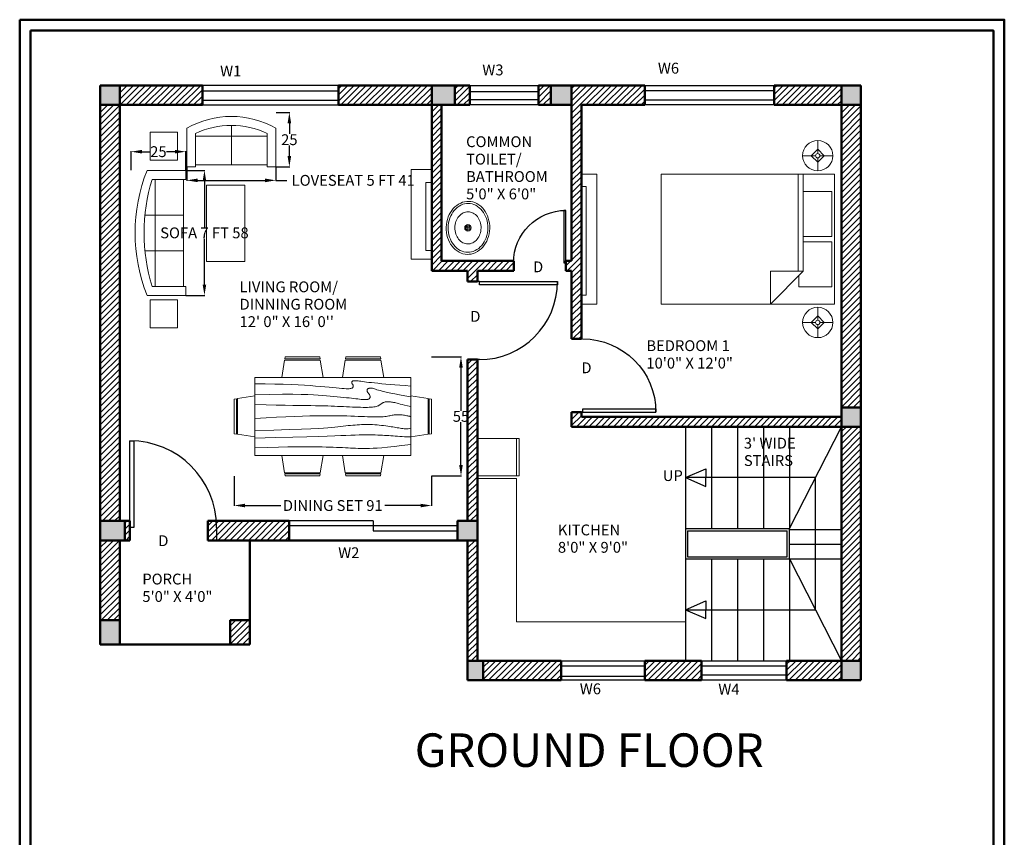
# Model space of a CAD drawing. Units: inches. Extents: x -25 to 429, y -18 to 847.
# Tile 3 of 3: x -25 to 429, y 470 to 847. Entities that reach past the tile are written whole.
import ezdxf

# ---------------------------------------------------------------- set-up
doc = ezdxf.new("R2010")
doc.units = ezdxf.units.IN
doc.header["$MEASUREMENT"] = 0
for name, color, linetype, lineweight in [('A-ANNO-DIMS', 2, 'Continuous', 18), ('A-ANNO-TEXT', 3, 'Continuous', 25), ('A-ANNO-TTLB', 7, 'Continuous', 50), ('A-AREA-IDEN', 7, 'Continuous', 25), ('A-DOOR', 4, 'Continuous', 25), ('A-FLOR-FIXT', 8, 'Continuous', 18), ('A-FLOR-STRS', 3, 'Continuous', 25), ('A-FURN', 8, 'Continuous', 18), ('A-GLAZ', 4, 'Continuous', 25), ('A-WALL', 7, 'Continuous', 50), ('A-WALL-FILL', 18, 'Continuous', 13), ('A-WALL-PATT', 252, 'Continuous', 13)]:
    doc.layers.add(name, color=color, linetype=linetype, lineweight=lineweight)
doc.styles.get("Standard").update_dxf_attribs({"font": 'arial.ttf'})
doc.dimstyles.get("Standard").update_dxf_attribs({"dimtxt": 5, "dimasz": 5, "dimexe": 0.18, "dimexo": 0.0625, "dimgap": 0.09, "dimtad": 0, "dimtih": 1, "dimtoh": 1, "dimdec": 1, "dimzin": 0, "dimdsep": 46, "dimlunit": 4, "dimtxsty": 'Standard', "dimcen": 0.09, "dimadec": 0, "dimazin": 0, "dimtfac": 1, "dimtdec": 1, "dimtofl": 0, "dimtmove": 0, "dimatfit": 3, "dimfxl": 1, "dimtolj": 1, "dimtzin": 0, "dimarcsym": 0})

# ---------------------------------------------------------------- blocks, each defined once
blk = doc.blocks.new('Sink - Oval top')
for p, q in [((-1, 0), (1, 0)), ((0, 1), (0, -1))]:
    blk.add_line(p, q)
for points in [[(-12.23, 0.39, 0.117634), (-11.46, -3.36, 0.104469), (-8.88, -6.8, 0.090016), (-5.08, -9.07, 0.08192), (-0.32, -10.02, 0.08192), (4.49, -9.38, 0.090016), (8.42, -7.36, 0.104469), (11.22, -4.09, 0.117634), (12.23, -0.39, 0.117634), (11.46, 3.36, 0.104469), (8.88, 6.8, 0.090016), (5.08, 9.07, 0.08192), (0.32, 10.02, 0.08192), (-4.49, 9.38, 0.090016), (-8.42, 7.36, 0.104469), (-11.22, 4.09, 0.117634)], [(-11.29, 0.16, 0.118622), (-10.52, -3.25, 0.104678), (-8.07, -6.36, 0.089562), (-4.54, -8.37, 0.081185), (-0.13, -9.15, 0.081185), (4.3, -8.49, 0.089562), (7.89, -6.58, 0.104678), (10.42, -3.55, 0.118622), (11.29, -0.16, 0.118622), (10.52, 3.25, 0.104678), (8.07, 6.36, 0.089562), (4.54, 8.37, 0.081185), (0.13, 9.15, 0.081185), (-4.3, 8.49, 0.089562), (-7.89, 6.58, 0.104678), (-10.42, 3.55, 0.118622)], [(-7.42, 0.08, 0.118283), (-6.91, -2.17, 0.104607), (-5.29, -4.21, 0.089718), (-2.97, -5.53, 0.081436), (-0.07, -6.04, 0.081436), (2.84, -5.59, 0.089718), (5.2, -4.33, 0.104607), (6.86, -2.32, 0.118283), (7.42, -0.08, 0.118283), (6.91, 2.17, 0.104607), (5.29, 4.21, 0.089718), (2.97, 5.53, 0.081436), (0.07, 6.04, 0.081436), (-2.84, 5.59, 0.089718), (-5.2, 4.33, 0.104607), (-6.86, 2.32, 0.118283)]]:
    blk.add_lwpolyline(points, format="xyb", close=True)
for radius in [1.5, 1]:
    blk.add_circle((0, 0), radius)
blk = doc.blocks.new('Bed - Queen')
for p, q in [((0, -80.00003), (0, 0)), ((0, 0), (59.99999, 0)), ((59.99999, 0), (59.99999, -80.00003)), ((7.99999, -1.2), (28.79998, -1.2)), ((7.99999, -14.4), (7.99999, -1.2)), ((28.79998, -1.2), (28.79998, -14.4)), ((31.19999, -1.2), (51.99999, -1.2)), ((31.19999, -14.4), (31.19999, -1.2)), ((51.99999, -1.2), (51.99999, -16.4)), ((0, -14.4), (44.8, -14.4)), ((44.8, -16.8), (0, -16.8)), ((59.99999, -29.6), (44.8, -14.4)), ((44.8, -14.4), (44.8, -29.6)), ((51.99999, -16.4), (46.79936, -16.4)), ((44.8, -29.6), (59.99999, -29.6)), ((59.99999, -80.00003), (0, -80.00003))]:
    blk.add_line(p, q)
blk = doc.blocks.new('Lamp - Table')
for p, q in [((0, 7), (0, 1)), ((-1, 0), (-7, 0)), ((0, 3), (-3, 0)), ((-3, 0), (0, -3)), ((3, 0), (0, 3)), ((0, -3), (3, 0)), ((1, 0), (7, 0)), ((0, -1), (0, -7))]:
    blk.add_line(p, q)
for radius in [7, 1]:
    blk.add_circle((0, 0), radius)
blk = doc.blocks.new('Sofa - Roundback 7 ft.')
for p, q in [((-12.00002, -32.4421), (-12.00003, -6.5971)), ((11.99997, -32.4421), (11.99998, -6.5971)), ((-36.000027, -34), (-36.000027, -11.4696)), ((35.99998, -34), (35.99998, -11.4696)), ((-35.999844, -13.3819), (35.9998, -13.3819)), ((-36.000027, -32.4421), (35.99998, -32.4421))]:
    blk.add_line(p, q)
for points in [[(-36.000027, -34), (-42.000027, -34), (-42.000027, -8)], [(41.99998, -8), (41.99998, -34), (35.99998, -34)]]:
    blk.add_lwpolyline(points)
for centre, radius, start, end in [((0, -114.25), 114.25, 68.43141, 111.5686), ((-0.00001, -127.1968), 121.1968, 72.72033, 107.2797)]:
    blk.add_arc(centre, radius, start, end)
blk = doc.blocks.new('Sofa - Roundback Loveseat 5 ft.')
for p, q in [((0, -32.44198), (0, -5.99998)), ((-24, -33.99998), (-24, -11.46958)), ((24.00004, -33.99998), (24.00004, -11.46958)), ((-23.9998, -13.38178), (23.99986, -13.38178)), ((-24, -32.44198), (24.00004, -32.44198))]:
    blk.add_line(p, q)
for points in [[(-24, -33.99998), (-30, -33.99998), (-30, -7.99998)], [(30.00004, -7.99998), (30.00004, -33.99998), (24.00004, -33.99998)]]:
    blk.add_lwpolyline(points)
for centre, radius, start, end in [((0, -60.24998), 60.24998, 60.13715, 119.8628), ((0, -61.38438), 55.38444, 64.32083, 115.6792)]:
    blk.add_arc(centre, radius, start, end)
blk = doc.blocks.new('Dining Set - 36 x 72 in.')
for p, q in [((-22, 27.5), (-22.1562, 26.50042)), ((-22, 27.5), (-6, 27.5)), ((-5.8437, 26.49966), (-6, 27.5)), ((6, 27.5), (5.8438, 26.50042)), ((6, 27.5), (22, 27.5)), ((22.1563, 26.49966), (22, 27.5)), ((-22.2343, 26.00059), (-23.4847, 17.99762)), ((-22.2304, 26), (-5.7608, 26)), ((-5.8416, 26.5), (-22.1534, 26.5)), ((-4.5152, 17.99762), (-5.7655, 25.99926)), ((5.7657, 26.00059), (4.5153, 17.99762)), ((5.7696, 26), (22.2392, 26)), ((22.1584, 26.5), (5.8466, 26.5)), ((23.4848, 17.99762), (22.2345, 25.99926)), ((36, 18), (-36, 18)), ((-36, 18), (-36, -18)), ((36, -18), (36, 18)), ((-44.0006, 8.23428), (-35.9976, 9.48474)), ((44.0006, 8.23428), (35.9976, 9.48474)), ((-45.5, 8), (-44.5004, 8.15617)), ((-45.5, 8), (-45.5, -8)), ((-44.5, -8.15843), (-44.5, 8.15338)), ((-44, 8.23041), (-44, -8.23915)), ((44, 8.23041), (44, -8.23915)), ((44.5, -8.15843), (44.5, 8.15338)), ((45.5, 8), (44.5005, 8.15617)), ((45.5, 8), (45.5, -8)), ((-44.4997, -8.15631), (-45.5, -8)), ((-35.9976, -9.48476), (-43.9993, -8.2345)), ((35.9976, -9.48476), (43.9993, -8.2345)), ((44.4997, -8.15631), (45.5, -8)), ((-36, -18), (36, -18)), ((-22.2343, -26.0006), (-23.4847, -17.99762)), ((-4.5152, -17.99762), (-5.7655, -25.99928)), ((5.7657, -26.0006), (4.5153, -17.99762)), ((23.4848, -17.99762), (22.2345, -25.99928)), ((-22.2304, -26), (-5.7608, -26)), ((-22, -27.5), (-22.1562, -26.50044)), ((-5.8416, -26.5), (-22.1534, -26.5)), ((-5.8437, -26.49967), (-6, -27.5)), ((5.7696, -26), (22.2392, -26)), ((6, -27.5), (5.8438, -26.50044)), ((22.1584, -26.5), (5.8466, -26.5)), ((22.1563, -26.49967), (22, -27.5)), ((-22, -27.5), (-6, -27.5)), ((6, -27.5), (22, -27.5))]:
    blk.add_line(p, q)
for points in [[(-36, 15), (-31.1772, 14.97754), (-26.8079, 14.91406), (-22.8538, 14.81543), (-19.276, 14.6875), (-16.0362, 14.53613), (-13.0957, 14.36718), (-10.4159, 14.18652), (-7.9583, 14), (-5.6904, 13.81315), (-3.6035, 13.63021), (-1.6954, 13.45508), (0.0365, 13.29166), (1.5945, 13.14388), (2.9811, 13.01562), (4.1988, 12.9108), (5.25, 12.83333), (6.1393, 12.78613), (6.8802, 12.76823), (7.4883, 12.77767), (7.9792, 12.8125), (8.3685, 12.87077), (8.6719, 12.95052), (8.9049, 13.0498), (9.0833, 13.16666), (9.2205, 13.29899), (9.3216, 13.44401), (9.3895, 13.59879), (9.4271, 13.76041), (9.4373, 13.92594), (9.4232, 14.09245), (9.3875, 14.257), (9.3333, 14.41666), (9.2638, 14.56917), (9.1836, 14.71484), (9.0975, 14.85465), (9.0104, 14.98958), (8.9272, 15.1206), (8.8529, 15.2487), (8.7922, 15.37483), (8.75, 15.5), (8.7305, 15.62467), (8.7344, 15.74739), (8.7617, 15.86621), (8.8125, 15.97916), (8.8867, 16.08431), (8.9844, 16.17968), (9.1055, 16.26334), (9.25, 16.33333), (9.4189, 16.38802), (9.6172, 16.42708), (9.8506, 16.45052), (10.125, 16.45833), (10.4463, 16.45052), (10.8203, 16.42708), (11.2529, 16.38802), (11.75, 16.33333), (12.3184, 16.26318), (12.9694, 16.17838), (13.7151, 16.07991), (14.5677, 15.96875), (15.5395, 15.84586), (16.6426, 15.71224), (17.8893, 15.56884), (19.2917, 15.41666), (20.859, 15.25667), (22.5879, 15.08984), (24.4721, 14.91715), (26.5052, 14.73958), (28.6809, 14.5581), (30.9929, 14.3737), (33.4347, 14.18733), (36, 14)], [(-36, 10), (-28.9766, 10.14274), (-23.1725, 10.20442), (-18.4241, 10.19775), (-14.5677, 10.13541), (-11.4399, 10.03011), (-8.877, 9.89453), (-6.7154, 9.74137), (-4.7917, 9.58333), (-2.9698, 9.43082), (-1.2246, 9.28515), (0.4415, 9.14534), (2.026, 9.01041), (3.5266, 8.87939), (4.9408, 8.7513), (6.266, 8.62516), (7.5, 8.5), (8.6411, 8.37549), (9.6914, 8.2539), (10.6538, 8.13818), (11.5312, 8.03125), (12.3267, 7.93603), (13.043, 7.85547), (13.6831, 7.79248), (14.25, 7.75), (14.7471, 7.7303), (15.1797, 7.73307), (15.5537, 7.75732), (15.875, 7.80208), (16.1494, 7.86637), (16.3828, 7.94922), (16.5811, 8.04964), (16.75, 8.16666), (16.8944, 8.29915), (17.0143, 8.44531), (17.1089, 8.60319), (17.1771, 8.77083), (17.218, 8.94629), (17.2305, 9.1276), (17.2137, 9.31282), (17.1667, 9.5), (17.0895, 9.6875), (16.987, 9.875), (16.8649, 10.0625), (16.7292, 10.25), (16.5856, 10.4375), (16.4401, 10.625), (16.2985, 10.8125), (16.1667, 11), (16.05, 11.18733), (15.9518, 11.3737), (15.8752, 11.5581), (15.8229, 11.73958), (15.798, 11.91715), (15.8034, 12.08984), (15.842, 12.25667), (15.9167, 12.41666), (16.0295, 12.56836), (16.1784, 12.70833), (16.3605, 12.83268), (16.5729, 12.9375), (16.8127, 13.01888), (17.0768, 13.07291), (17.3625, 13.0957), (17.6667, 13.08333), (17.9894, 13.03312), (18.3418, 12.94726), (18.7382, 12.82918), (19.1927, 12.68229), (19.7195, 12.51001), (20.3327, 12.31575), (21.0465, 12.10294), (21.875, 11.875), (22.8357, 11.63354), (23.959, 11.37304), (25.2786, 11.08618), (26.8282, 10.76562), (28.6414, 10.40405), (30.752, 9.99414), (33.1936, 9.52856), (36, 9)], [(-36, 5.5), (-30.7157, 5.3348), (-26.069, 5.20963), (-21.9946, 5.11767), (-18.4271, 5.05208), (-15.3009, 5.00602), (-12.5508, 4.97265), (-10.1112, 4.94515), (-7.9167, 4.91666), (-5.909, 4.88167), (-4.0586, 4.83984), (-2.3429, 4.79215), (-0.7396, 4.73958), (0.7739, 4.6831), (2.22, 4.6237), (3.6213, 4.56233), (5, 4.5), (6.373, 4.43782), (7.7344, 4.3776), (9.0723, 4.32129), (10.375, 4.27083), (11.6309, 4.22819), (12.8281, 4.19531), (13.9551, 4.17415), (15, 4.16666), (15.954, 4.17448), (16.819, 4.19791), (17.6001, 4.23698), (18.3021, 4.29166), (18.9299, 4.36198), (19.4883, 4.44791), (19.9823, 4.54948), (20.4167, 4.66666), (20.7969, 4.79899), (21.1302, 4.94401), (21.4245, 5.09879), (21.6875, 5.26041), (21.9271, 5.42594), (22.1511, 5.59245), (22.3672, 5.757), (22.5834, 5.91666), (22.8065, 6.06868), (23.0404, 6.21093), (23.2879, 6.34147), (23.5521, 6.45833), (23.8358, 6.55957), (24.142, 6.64323), (24.4735, 6.70735), (24.8334, 6.75), (25.2235, 6.76969), (25.642, 6.76692), (26.0858, 6.74267), (26.5521, 6.69791), (27.0379, 6.63362), (27.5404, 6.55078), (28.0565, 6.45036), (28.5834, 6.33333), (29.1242, 6.19987), (29.7071, 6.04687), (30.3661, 5.87044), (31.1354, 5.66666), (32.0493, 5.43164), (33.142, 5.16146), (34.4475, 4.85221), (36, 4.5)], [(-36, -1), (-30.7915, -0.6591), (-26.0195, -0.38216), (-21.6519, -0.16284), (-17.6563, 0.00521), (-14.0005, 0.12833), (-10.6523, 0.21289), (-7.5796, 0.26522), (-4.75, 0.29166), (-2.134, 0.29793), (0.2878, 0.28711), (2.5317, 0.26163), (4.6146, 0.22396), (6.5529, 0.17651), (8.3633, 0.12174), (10.0623, 0.06209), (11.6667, 0), (13.1899, -0.06201), (14.6341, -0.1211), (15.9982, -0.17432), (17.2813, -0.21875), (18.4823, -0.25147), (19.6003, -0.26953), (20.6343, -0.27002), (21.5834, -0.25), (22.4481, -0.20768), (23.2357, -0.14584), (23.9549, -0.06836), (24.6146, 0.02083), (25.2235, 0.11784), (25.7904, 0.21875), (26.3241, 0.31966), (26.8334, 0.41666), (27.3265, 0.50618), (27.8099, 0.58593), (28.2894, 0.65397), (28.7709, 0.70833), (29.2601, 0.74707), (29.763, 0.76823), (30.2855, 0.76985), (30.8334, 0.75), (31.4088, 0.70784), (31.9994, 0.64713), (32.589, 0.57275), (33.1615, 0.48958), (33.7008, 0.4025), (34.1908, 0.3164), (34.6153, 0.23616), (34.9584, 0.16666), (35.2099, 0.11165), (35.3848, 0.07031), (35.504, 0.04069), (35.5886, 0.02083), (35.6594, 0.00879), (35.7377, 0.0026), (35.8442, 0.00032), (36, 0)], [(-36, -6.5), (-27.1843, -6.31267), (-20.084, -6.1263), (-14.469, -5.9419), (-10.1094, -5.76042), (-6.7752, -5.58285), (-4.2363, -5.41016), (-2.2629, -5.24333), (-0.625, -5.08334), (0.8708, -4.93099), (2.2715, -4.78646), (3.5872, -4.64974), (4.8281, -4.52084), (6.0046, -4.39974), (7.127, -4.28646), (8.2053, -4.18099), (9.25, -4.08334), (10.2705, -3.99382), (11.2734, -3.91407), (12.2647, -3.84603), (13.25, -3.79167), (14.2354, -3.75293), (15.2266, -3.73177), (16.2295, -3.73015), (17.25, -3.75), (18.2912, -3.79248), (19.3451, -3.85547), (20.4009, -3.93604), (21.4479, -4.03125), (22.4754, -4.13819), (23.4727, -4.25391), (24.4289, -4.37549), (25.3334, -4.5), (26.1785, -4.62492), (26.9694, -4.74935), (27.7145, -4.87281), (28.4219, -4.99479), (29.1, -5.11483), (29.7572, -5.23242), (30.4016, -5.34709), (31.0417, -5.45834), (31.6837, -5.56437), (32.3262, -5.65821), (32.9658, -5.73153), (33.599, -5.77604), (34.2224, -5.78345), (34.8327, -5.74545), (35.4264, -5.65373), (36, -5.5)], [(-36, -10), (-26.4022, -9.81299), (-18.4675, -9.62891), (-11.9839, -9.45069), (-6.7396, -9.28125), (-2.5226, -9.12354), (0.8789, -8.98047), (3.6769, -8.85498), (6.0833, -8.75), (8.2767, -8.66765), (10.3021, -8.60677), (12.1712, -8.56543), (13.8958, -8.54167), (15.4876, -8.53353), (16.9583, -8.53907), (18.3197, -8.55632), (19.5834, -8.58334), (20.7616, -8.61841), (21.8685, -8.66081), (22.9188, -8.71004), (23.9271, -8.76563), (24.9081, -8.82707), (25.8763, -8.89388), (26.8465, -8.96558), (27.8334, -9.04167), (28.8474, -9.12118), (29.8828, -9.20117), (30.93, -9.27824), (31.9792, -9.34896), (33.0205, -9.40991), (34.0443, -9.45768), (35.0407, -9.48885), (36, -9.5)], [(-36, -14.5), (-30.0881, -14.33513), (-25.0332, -14.21224), (-20.7312, -14.12647), (-17.0781, -14.07292), (-13.97, -14.04671), (-11.3027, -14.04297), (-8.9724, -14.05681), (-6.875, -14.08334), (-4.9224, -14.11833), (-3.0905, -14.16016), (-1.3709, -14.20785), (0.2448, -14.26042), (1.7647, -14.3169), (3.1973, -14.3763), (4.5507, -14.43767), (5.8333, -14.5), (7.0554, -14.5621), (8.235, -14.62175), (9.3922, -14.67652), (10.5469, -14.72396), (11.7192, -14.76164), (12.929, -14.78711), (14.1965, -14.79794), (15.5417, -14.79167), (16.9933, -14.76424), (18.6152, -14.70508), (20.4804, -14.60197), (22.6615, -14.44271), (25.2312, -14.21509), (28.2624, -13.9069), (31.8277, -13.50594), (36, -13)]]:
    blk.add_lwpolyline(points)
blk = doc.blocks.new('*U10')
for p, q in [((0, 0), (0, -6)), ((40, 0), (40, -6))]:
    blk.add_line(p, q)
blk.add_lwpolyline([(0, 0), (0, 40), (1.75, 40), (1.75, 0)], close=True)
blk.add_arc((0, 0), 40, 0, 90)
blk = doc.blocks.new('*D21')
at = {"layer": 'A-ANNO-DIMS', "color": 0, "lineweight": -2, "ltscale": 0.5, "transparency": 16777216}
for p, q in [((51.61, 777.34), (60.37, 777.34)), ((60.19, 772.34), (60.19, 751.19)), ((60.19, 724.68), (60.19, 745.83)), ((51.61, 719.68), (60.37, 719.68))]:
    blk.add_line(p, q, dxfattribs=at)
at = {"layer": 'A-ANNO-DIMS', "color": 0, "lineweight": 100, "ltscale": 0.5, "transparency": 16777216}
for points in [[(59.36, 772.34), (61.03, 772.34), (60.19, 777.34)], [(59.36, 724.68), (61.03, 724.68), (60.19, 719.68)]]:
    blk.add_solid(points, dxfattribs=at)
at = {"layer": 'Defpoints', "color": 0, "lineweight": 100, "ltscale": 0.5, "transparency": 16777216}
for p in [(51.54, 777.34), (60.19, 777.34), (51.54, 719.68)]:
    blk.add_point(p, dxfattribs=at)
at = {"layer": 'A-ANNO-DIMS', "color": 0, "ltscale": 0.5, "transparency": 16777216, "insert": (60.19, 748.51), "char_height": 5, "attachment_point": 5}
blk.add_mtext('\\A1;SOFA 7 FT 58', dxfattribs=at)
blk = doc.blocks.new('*D22')
at = {"layer": 'A-ANNO-DIMS', "color": 0, "lineweight": -2, "ltscale": 0.5, "transparency": 16777216}
for p, q in [((26.37, 777.4), (26.37, 786.17)), ((51.54, 777.4), (51.54, 786.17)), ((31.37, 785.99), (35.23, 785.99)), ((46.54, 785.99), (42.69, 785.99))]:
    blk.add_line(p, q, dxfattribs=at)
at = {"layer": 'A-ANNO-DIMS', "color": 0, "lineweight": 100, "ltscale": 0.5, "transparency": 16777216}
for points in [[(31.37, 786.82), (31.37, 785.15), (26.37, 785.99)], [(46.54, 786.82), (46.54, 785.15), (51.54, 785.99)]]:
    blk.add_solid(points, dxfattribs=at)
at = {"layer": 'Defpoints', "color": 0, "lineweight": 100, "ltscale": 0.5, "transparency": 16777216}
for p in [(26.37, 785.99), (26.37, 777.34), (51.54, 777.34)]:
    blk.add_point(p, dxfattribs=at)
at = {"layer": 'A-ANNO-DIMS', "color": 0, "ltscale": 0.5, "transparency": 16777216, "insert": (38.96, 785.99), "char_height": 5, "attachment_point": 5}
blk.add_mtext('\\A1;25', dxfattribs=at)
blk = doc.blocks.new('*D25')
at = {"layer": 'A-ANNO-DIMS', "color": 0, "lineweight": -2, "ltscale": 0.5, "transparency": 16777216}
for p, q in [((52.02, 778.86), (52.02, 772.57)), ((93.2, 778.86), (93.2, 772.57)), ((57.02, 772.75), (88.2, 772.75)), ((93.2, 772.75), (98.2, 772.75))]:
    blk.add_line(p, q, dxfattribs=at)
at = {"layer": 'A-ANNO-DIMS', "color": 0, "lineweight": 100, "ltscale": 0.5, "transparency": 16777216}
for points in [[(57.02, 773.58), (57.02, 771.91), (52.02, 772.75)], [(88.2, 773.58), (88.2, 771.91), (93.2, 772.75)]]:
    blk.add_solid(points, dxfattribs=at)
at = {"layer": 'Defpoints', "color": 0, "lineweight": 100, "ltscale": 0.5, "transparency": 16777216}
for p in [(52.02, 778.93), (93.2, 778.93), (93.2, 772.75)]:
    blk.add_point(p, dxfattribs=at)
at = {"layer": 'A-ANNO-DIMS', "color": 0, "ltscale": 0.5, "transparency": 16777216, "insert": (128.84, 772.75), "char_height": 5, "attachment_point": 5}
blk.add_mtext('\\A1;LOVESEAT 5 FT 41', dxfattribs=at)
blk = doc.blocks.new('*D26')
at = {"layer": 'A-ANNO-DIMS', "color": 0, "lineweight": -2, "ltscale": 0.5, "transparency": 16777216}
for p, q in [((93.27, 804.1), (99.56, 804.1)), ((99.38, 799.1), (99.38, 794.15)), ((99.38, 783.93), (99.38, 788.87)), ((93.27, 778.93), (99.56, 778.93))]:
    blk.add_line(p, q, dxfattribs=at)
at = {"layer": 'A-ANNO-DIMS', "color": 0, "lineweight": 100, "ltscale": 0.5, "transparency": 16777216}
for points in [[(98.55, 799.1), (100.21, 799.1), (99.38, 804.1)], [(98.55, 783.93), (100.21, 783.93), (99.38, 778.93)]]:
    blk.add_solid(points, dxfattribs=at)
at = {"layer": 'Defpoints', "color": 0, "lineweight": 100, "ltscale": 0.5, "transparency": 16777216}
for p in [(93.2, 804.1), (99.38, 804.1), (93.2, 778.93)]:
    blk.add_point(p, dxfattribs=at)
at = {"layer": 'A-ANNO-DIMS', "color": 0, "ltscale": 0.5, "transparency": 16777216, "insert": (99.38, 791.51), "char_height": 5, "attachment_point": 5}
blk.add_mtext('\\A1;25', dxfattribs=at)
blk = doc.blocks.new('*D35')
at = {"layer": 'A-ANNO-DIMS', "color": 0, "lineweight": -2, "ltscale": 0.5, "transparency": 16777216}
for p, q in [((73.92, 636.24), (73.92, 622.48)), ((164.92, 636.24), (164.92, 622.48)), ((78.92, 622.66), (95.4, 622.66)), ((159.92, 622.66), (143.44, 622.66))]:
    blk.add_line(p, q, dxfattribs=at)
at = {"layer": 'A-ANNO-DIMS', "color": 0, "lineweight": 100, "ltscale": 0.5, "transparency": 16777216}
for points in [[(78.92, 623.49), (78.92, 621.82), (73.92, 622.66)], [(159.92, 623.49), (159.92, 621.82), (164.92, 622.66)]]:
    blk.add_solid(points, dxfattribs=at)
at = {"layer": 'Defpoints', "color": 0, "lineweight": 100, "ltscale": 0.5, "transparency": 16777216}
for p in [(73.92, 636.31), (164.92, 636.31), (164.92, 622.66)]:
    blk.add_point(p, dxfattribs=at)
at = {"layer": 'A-ANNO-DIMS', "color": 0, "ltscale": 0.5, "transparency": 16777216, "insert": (119.42, 622.66), "char_height": 5, "attachment_point": 5}
blk.add_mtext('\\A1;DINING SET 91', dxfattribs=at)
blk = doc.blocks.new('*D36')
at = {"layer": 'A-ANNO-DIMS', "color": 0, "lineweight": -2, "ltscale": 0.5, "transparency": 16777216}
for p, q in [((164.98, 691.31), (178.75, 691.31)), ((178.57, 686.31), (178.57, 666.44)), ((178.57, 641.31), (178.57, 661.17)), ((164.98, 636.31), (178.75, 636.31))]:
    blk.add_line(p, q, dxfattribs=at)
at = {"layer": 'A-ANNO-DIMS', "color": 0, "lineweight": 100, "ltscale": 0.5, "transparency": 16777216}
for points in [[(177.73, 686.31), (179.4, 686.31), (178.57, 691.31)], [(177.73, 641.31), (179.4, 641.31), (178.57, 636.31)]]:
    blk.add_solid(points, dxfattribs=at)
at = {"layer": 'Defpoints', "color": 0, "lineweight": 100, "ltscale": 0.5, "transparency": 16777216}
for p in [(164.92, 691.31), (178.57, 691.31), (164.92, 636.31)]:
    blk.add_point(p, dxfattribs=at)
at = {"layer": 'A-ANNO-DIMS', "color": 0, "ltscale": 0.5, "transparency": 16777216, "insert": (178.57, 663.81), "char_height": 5, "attachment_point": 5}
blk.add_mtext('\\A1;55', dxfattribs=at)

msp = doc.modelspace()

# ---------------------------------------------------------------- hatches: boundary and pattern name
at = {"layer": 'A-WALL-FILL', "ltscale": 0.5}
h = msp.add_hatch(color=256, dxfattribs=at)
h.dxf.hatch_style = 1
h.paths.add_polyline_path([(21.13, 816.54), (12.13, 816.54), (12.13, 807.54), (21.13, 807.54)])
h.paths.add_polyline_path([(175.79, 816.54), (165.13, 816.54), (165.13, 807.54), (175.79, 807.54)])
h.paths.add_polyline_path([(229.63, 816.54), (220.08, 816.54), (220.08, 807.54), (229.63, 807.54)])
h.paths.add_polyline_path([(363.13, 816.54), (354.13, 816.54), (354.13, 807.54), (357.13, 807.54), (363.13, 807.54)])
h.paths.add_polyline_path([(186.13, 615.54), (176.99, 615.54), (176.99, 606.54), (186.13, 606.54)])
h.paths.add_polyline_path([(23.44, 615.54), (12.13, 615.54), (12.13, 606.54), (23.44, 606.54)])
h.paths.add_polyline_path([(21.13, 569.73), (12.13, 569.73), (12.13, 558.54), (21.13, 558.54)])
h.paths.add_polyline_path([(188.77, 551.04), (181.63, 551.04), (181.63, 542.04), (188.77, 542.04)])
h.paths.add_polyline_path([(363.13, 551.04), (354.13, 551.04), (354.13, 542.04), (363.13, 542.04)])
h.paths.add_polyline_path([(363.13, 667.89), (354.13, 667.89), (354.13, 659.04), (363.13, 659.04)])
at = {"layer": 'A-WALL-PATT', "ltscale": 0.5}
h = msp.add_hatch(dxfattribs=at)
h.set_pattern_fill('ANSI31', color=256, scale=16)
h.paths.add_polyline_path([(21.13, 807.54), (12.13, 807.54), (12.13, 615.54), (21.13, 615.54)])
h.paths.add_polyline_path([(59.28, 816.54), (21.13, 816.54), (21.13, 807.54), (59.28, 807.54)])
h.paths.add_polyline_path([(165.13, 816.54), (122.04, 816.54), (122.04, 807.54), (165.13, 807.54)])
h.paths.add_polyline_path([(182.62, 816.54), (175.79, 816.54), (175.79, 807.54), (182.62, 807.54)])
h.paths.add_polyline_path([(220.08, 816.54), (214.31, 816.54), (214.31, 807.54), (220.08, 807.54)])
h.paths.add_polyline_path([(263.36, 816.54), (229.63, 816.54), (229.63, 807.54), (229.63, 735.54), (227.02, 735.54), (227.02, 731.04), (229.63, 731.04), (229.63, 699.54), (234.13, 699.54), (234.13, 807.54), (263.36, 807.54)])
h.paths.add_polyline_path([(169.63, 807.54), (165.13, 807.54), (165.13, 731.04), (181.63, 731.04), (181.63, 726.06), (186.13, 726.06), (186.13, 731.04), (203.02, 731.04), (203.02, 735.54), (169.63, 735.54)])
h.paths.add_polyline_path([(354.13, 816.54), (323.12, 816.54), (323.12, 807.54), (354.13, 807.54)])
h.paths.add_polyline_path([(363.13, 807.54), (354.13, 807.54), (354.13, 667.89), (363.13, 667.89)])
h.paths.add_polyline_path([(354.13, 663.54), (234.13, 663.54), (234.13, 665.73), (229.63, 665.73), (229.63, 659.04), (354.13, 659.04)])
h.paths.add_polyline_path([(363.13, 659.04), (354.13, 659.04), (354.13, 612.04), (354.13, 598.04), (354.13, 551.04), (363.13, 551.04)])
h.paths.add_polyline_path([(354.13, 551.04), (328.82, 551.04), (328.82, 542.04), (354.13, 542.04)])
h.paths.add_polyline_path([(289.58, 551.04), (263.34, 551.04), (263.34, 542.04), (289.58, 542.04)])
h.paths.add_polyline_path([(224.82, 551.04), (188.77, 551.04), (188.77, 542.04), (224.82, 542.04)])
h.paths.add_polyline_path([(186.13, 606.54), (181.63, 606.54), (181.63, 551.04), (186.13, 551.04)])
h.paths.add_polyline_path([(99.25, 615.54), (61.79, 615.54), (61.79, 606.54), (99.25, 606.54)])
h.paths.add_polyline_path([(81.13, 569.73), (72.13, 569.73), (72.13, 558.54), (81.13, 558.54)])
h.paths.add_polyline_path([(21.13, 606.54), (12.13, 606.54), (12.13, 569.73), (21.13, 569.73)])
h.paths.add_polyline_path([(25.79, 615.54), (23.44, 615.54), (23.44, 606.54), (25.79, 606.54)])
h.paths.add_polyline_path([(186.13, 690.06), (181.63, 690.06), (181.63, 615.54), (186.13, 615.54)])

# ---------------------------------------------------------------- linework, layer by layer
at = {"layer": 'A-ANNO-TTLB', "ltscale": 0.5}
for points in [[(-25.05, 846.91), (429.28, 846.91), (429.28, -17.53), (-25.05, -17.53)], [(-20.05, 841.91), (424.28, 841.91), (424.28, -12.53), (-20.05, -12.53)]]:
    msp.add_lwpolyline(points, close=True, dxfattribs=at)
at = {"layer": 'A-FLOR-FIXT', "ltscale": 0.5}
for p, q in [((204.13, 653.62), (205.46, 653.62)), ((205.46, 653.62), (205.46, 636.32)), ((205.46, 636.32), (204.13, 636.32)), ((186.13, 635.19), (204.13, 635.19)), ((204.13, 635.19), (204.13, 569.04)), ((204.13, 569.04), (282.13, 569.04))]:
    msp.add_line(p, q, dxfattribs=at)
msp.add_lwpolyline([(186.13, 636.37), (204.13, 636.37), (204.13, 653.62), (186.13, 653.62)], close=True, dxfattribs=at)
at = {"layer": 'A-FLOR-STRS'}
for p, q in [((282.13, 659.04), (282.13, 612.04)), ((282.13, 612.04), (282.13, 598.04)), ((283.13, 611.04), (283.13, 599.04)), ((282.13, 598.04), (282.13, 551.04))]:
    msp.add_line(p, q, dxfattribs=at)
at = {"layer": 'A-FLOR-STRS', "ltscale": 0.5}
for p, q in [((294.12, 659.04), (294.12, 612.04)), ((306.12, 659.04), (306.12, 612.04)), ((318.12, 659.04), (318.12, 612.04)), ((330.12, 659.04), (330.12, 612.04)), ((330.13, 612.04), (354.13, 659.04)), ((282.13, 635.54), (291.57, 639.63)), ((291.57, 639.63), (291.57, 635.54)), ((342.13, 635.54), (282.13, 635.54)), ((282.13, 635.54), (291.57, 631.46)), ((291.57, 631.46), (291.57, 635.54)), ((342.12, 574.54), (342.13, 635.54)), ((282.13, 612.04), (330.13, 612.04)), ((283.13, 611.04), (329.13, 611.04)), ((329.13, 599.04), (329.13, 611.04)), ((330.13, 599.04), (330.13, 612.04)), ((330.13, 611.04), (330.13, 612.04)), ((330.13, 611.54), (354.13, 611.54)), ((330.13, 604.88), (354.13, 604.88)), ((282.13, 598.04), (330.13, 598.04)), ((282.13, 598.04), (282.13, 551.04)), ((283.13, 599.04), (329.13, 599.04)), ((294.12, 598.04), (294.12, 551.04)), ((306.12, 598.04), (306.12, 551.04)), ((318.12, 598.04), (318.12, 551.04)), ((330.12, 598.04), (330.12, 551.04)), ((330.12, 598.04), (354.13, 551.04)), ((330.13, 598.04), (330.13, 599.04)), ((330.13, 598.04), (354.13, 598.04)), ((282.13, 574.54), (291.57, 578.63)), ((291.57, 578.63), (291.57, 574.54)), ((282.13, 574.54), (342.12, 574.54)), ((282.13, 574.54), (291.57, 570.46)), ((291.57, 570.46), (291.57, 574.54))]:
    msp.add_line(p, q, dxfattribs=at)
at = {"layer": 'A-FURN'}
for points in [[(47.84, 782.11), (35.08, 782.11), (35.08, 794.96), (47.84, 794.96)], [(78.87, 735.31), (61.13, 735.31), (61.13, 770.47), (78.87, 770.47)], [(47.84, 704.68), (35.08, 704.68), (35.08, 717.53), (47.84, 717.53)]]:
    msp.add_lwpolyline(points, close=True, dxfattribs=at)
at = {"layer": 'A-FURN', "ltscale": 0.5}
for points in [[(165.13, 736.45), (155.55, 736.45), (155.55, 777.77), (165.13, 777.77)], [(234.13, 775.57), (241.21, 775.57), (241.21, 715.57), (234.13, 715.57)], [(165.13, 771.71), (162.28, 771.71), (162.28, 740.34), (165.13, 740.34)], [(234.13, 769.95), (236.36, 769.95), (236.36, 719.82), (234.13, 719.82)]]:
    msp.add_lwpolyline(points, close=True, dxfattribs=at)
at = {"layer": 'A-GLAZ', "ltscale": 0.5}
for p, q in [((99.25, 615.54), (99.25, 611.04)), ((138.12, 615.54), (99.25, 615.54)), ((99.25, 615.54), (99.25, 611.04)), ((99.25, 613.37), (138.12, 613.37)), ((138.12, 615.54), (138.12, 611.04)), ((138.12, 613.37), (176.99, 613.37)), ((138.12, 611.04), (176.99, 611.04))]:
    msp.add_line(p, q, dxfattribs=at)
for points in [[(59.28, 807.54), (122.04, 807.54), (122.04, 816.54), (59.28, 816.54)], [(59.28, 814.03), (122.04, 814.03), (122.04, 809.61), (59.28, 809.61)], [(182.62, 816.54), (214.31, 816.54), (214.31, 807.54), (182.62, 807.54)], [(182.62, 813.72), (214.31, 813.72), (214.31, 809.89), (182.62, 809.89)], [(263.36, 816.54), (323.12, 816.54), (323.12, 807.54), (263.36, 807.54)], [(263.36, 814.23), (323.12, 814.23), (323.12, 809.71), (263.36, 809.71)], [(224.82, 551.04), (263.34, 551.04), (263.34, 542.04), (224.82, 542.04)], [(289.58, 551.04), (328.82, 551.04), (328.82, 542.04), (289.58, 542.04)], [(224.82, 548.67), (263.34, 548.67), (263.34, 543.82), (224.82, 543.82)], [(289.58, 548.72), (328.82, 548.72), (328.82, 544.4), (289.58, 544.4)]]:
    msp.add_lwpolyline(points, close=True, dxfattribs=at)
at = {"layer": 'A-WALL'}
for p, q in [((12.13, 816.54), (12.13, 558.54)), ((59.28, 816.54), (12.13, 816.54)), ((21.13, 816.54), (21.13, 615.54)), ((182.62, 816.54), (122.04, 816.54)), ((165.13, 816.54), (165.13, 731.04)), ((263.36, 816.54), (214.31, 816.54)), ((229.63, 816.54), (229.63, 735.54)), ((363.13, 816.54), (323.12, 816.54)), ((354.13, 816.54), (354.13, 663.54)), ((363.13, 816.54), (363.13, 542.04)), ((59.28, 807.54), (12.13, 807.54)), ((165.13, 807.54), (122.04, 807.54)), ((169.63, 807.54), (169.63, 735.54)), ((182.62, 807.54), (169.63, 807.54)), ((182.62, 807.54), (171.13, 807.54)), ((229.63, 807.54), (214.31, 807.54)), ((229.63, 807.54), (214.31, 807.54)), ((234.13, 807.54), (234.13, 699.54)), ((263.36, 807.54), (234.13, 807.54)), ((363.13, 807.54), (323.12, 807.54)), ((357.13, 807.54), (354.13, 807.54)), ((203.02, 735.54), (169.63, 735.54)), ((203.02, 735.54), (203.02, 731.04)), ((229.63, 735.54), (227.02, 735.54)), ((227.02, 731.04), (227.02, 735.54)), ((181.63, 731.04), (165.13, 731.04)), ((181.63, 731.04), (181.63, 726.06)), ((186.13, 731.04), (186.13, 726.06)), ((203.02, 731.04), (186.13, 731.04)), ((229.63, 731.04), (227.02, 731.04)), ((229.63, 731.04), (229.63, 699.54)), ((186.13, 726.06), (181.63, 726.06)), ((234.13, 699.54), (229.63, 699.54)), ((181.63, 690.06), (186.13, 690.06)), ((181.63, 690.06), (181.63, 615.54)), ((186.13, 690.06), (186.13, 551.04)), ((229.63, 665.73), (229.63, 659.04)), ((234.13, 665.73), (234.13, 663.54)), ((354.13, 663.54), (234.13, 663.54)), ((363.13, 659.04), (229.63, 659.04)), ((354.13, 659.04), (354.13, 612.04)), ((25.79, 615.54), (12.13, 615.54)), ((25.79, 606.54), (25.79, 615.54)), ((61.79, 615.54), (61.79, 606.54)), ((99.25, 615.54), (61.79, 615.54)), ((181.63, 615.54), (176.99, 615.54)), ((354.13, 612.04), (354.13, 598.04)), ((25.79, 606.54), (12.13, 606.54)), ((21.13, 606.54), (21.13, 558.54)), ((181.63, 606.54), (61.79, 606.54)), ((181.63, 606.54), (181.63, 542.04)), ((354.13, 598.04), (354.13, 542.04)), ((12.13, 558.54), (21.13, 558.54)), ((224.82, 551.04), (186.13, 551.04)), ((289.58, 551.04), (263.34, 551.04)), ((363.13, 551.04), (328.82, 551.04)), ((224.82, 542.04), (186.13, 542.04)), ((289.58, 542.04), (263.34, 542.04)), ((363.13, 542.04), (328.82, 542.04))]:
    msp.add_line(p, q, dxfattribs=at)
at = {"layer": 'A-WALL', "ltscale": 0.5}
for p, q in [((59.28, 807.54), (59.28, 816.54)), ((122.04, 807.54), (122.04, 816.54)), ((182.62, 816.54), (182.62, 807.54)), ((214.31, 816.54), (214.31, 807.54)), ((263.36, 816.54), (263.36, 807.54)), ((323.12, 816.54), (323.12, 807.54)), ((234.13, 665.73), (229.63, 665.73)), ((99.25, 615.54), (99.25, 606.54)), ((81.13, 558.54), (81.13, 606.54)), ((21.13, 558.54), (81.13, 558.54)), ((224.82, 551.04), (224.82, 542.04)), ((263.34, 551.04), (263.34, 542.04)), ((289.58, 551.04), (289.58, 542.04)), ((328.82, 551.04), (328.82, 542.04))]:
    msp.add_line(p, q, dxfattribs=at)
for points in [[(165.13, 816.54), (175.79, 816.54), (175.79, 807.54), (165.13, 807.54)], [(229.63, 807.54), (220.08, 807.54), (220.08, 816.54), (229.63, 816.54)], [(354.13, 659.04), (363.13, 659.04), (363.13, 667.89), (354.13, 667.89)], [(12.13, 615.54), (23.44, 615.54), (23.44, 606.54), (12.13, 606.54)], [(186.13, 606.54), (176.99, 606.54), (176.99, 615.54), (186.13, 615.54)], [(21.13, 558.54), (12.13, 558.54), (12.13, 569.73), (21.13, 569.73)], [(81.13, 558.54), (72.13, 558.54), (72.13, 569.73), (81.13, 569.73)], [(181.63, 542.04), (188.77, 542.04), (188.77, 551.04), (181.63, 551.04)]]:
    msp.add_lwpolyline(points, close=True, dxfattribs=at)

# ---------------------------------------------------------------- block references
at = {"layer": 'A-DOOR', "xscale": -0.6051608708458737, "yscale": 0.6051608708458737, "zscale": 0.6051608708458737}
msp.add_blockref('*U10', (227.02, 734.68), dxfattribs=at)
at = {"layer": 'A-DOOR', "rotation": 270}
for p, xscale, yscale, zscale in [((187.04, 726.06), 0.9017801120568154, 0.9017801120568154, 0.9017801120568154), ((234.7, 665.73), -0.8456826360449525, 0.8456826360449525, 0.8456826360449525)]:
    msp.add_blockref('*U10', p, dxfattribs=dict(at, xscale=xscale, yscale=yscale, zscale=zscale))
at = {"layer": 'A-DOOR'}
msp.add_blockref('*U10', (25.79, 612.54), dxfattribs=at)
at = {"layer": 'A-FLOR-FIXT', "rotation": 90}
msp.add_blockref('Sink - Oval top', (181.8, 750.82), dxfattribs=at)
at = {"layer": 'A-FURN', "xscale": 0.6864333361151705, "yscale": 0.6864333361151705, "zscale": 0.6864333361151705}
msp.add_blockref('Sofa - Roundback Loveseat 5 ft.', (72.61, 802.26), dxfattribs=at)
at = {"layer": 'A-FURN', "rotation": 270}
for name, p in [('Lamp - Table', (343.19, 784.14)), ('Bed - Queen', (350.93, 775.57)), ('Lamp - Table', (343.19, 707.15))]:
    msp.add_blockref(name, p, dxfattribs=at)
at = {"layer": 'A-FURN', "xscale": 0.6864333361151705, "yscale": 0.6864333361151705, "zscale": 0.6864333361151705, "rotation": 89.99999999999999}
msp.add_blockref('Sofa - Roundback 7 ft.', (28.2, 748.51), dxfattribs=at)
at = {"layer": 'A-FURN', "ltscale": 0.5}
msp.add_blockref('Dining Set - 36 x 72 in.', (119.42, 663.81), dxfattribs=at)

# ---------------------------------------------------------------- texts
at = {"layer": 'A-ANNO-TEXT', "ltscale": 0.5}
for s, height, p in [('W6', 5, (269.44, 822.03)), ('W1', 5, (67.43, 820.7)), ('W3', 5, (188.41, 821.21)), ('D', 5, (211.83, 730.33)), ('D', 5, (182.87, 707.47)), ('D', 5, (234.13, 683.73)), ("3' WIDE", 5, (309.09, 648.95)), ('STAIRS', 5, (309.09, 640.92)), ('UP', 5, (271.69, 633.98)), ('D', 5, (38.9, 603.91)), ('W2', 5, (121.92, 598.37)), ('W6', 5, (233.39, 535.55)), ('W4', 5, (297.31, 535.39)), ('GROUND FLOOR', 15.4568, (157.23, 502.03))]:
    msp.add_text(s, height=height, dxfattribs=at).set_placement(p)
at = {"layer": 'A-AREA-IDEN', "ltscale": 0.5}
for s, p in [('COMMON', (180.93, 788.08)), ('TOILET/', (180.93, 780.05)), ('BATHROOM', (180.93, 772.01)), ('5\'0" X 6\'0"', (180.93, 763.98)), ('LIVING ROOM/ ', (76.39, 721.1)), ('DINNING ROOM', (76.39, 713.07)), ('12\' 0" X 16\' 0\'\'', (76.39, 705.04)), ('BEDROOM 1', (264.11, 693.94)), ('10\'0" X 12\'0"', (264.11, 685.9)), ('KITCHEN', (223.28, 608.9)), ('8\'0" X 9\'0"', (223.28, 600.87)), ('PORCH', (31.53, 586.22)), ('5\'0" X 4\'0"', (31.53, 578.18))]:
    msp.add_text(s, height=5, dxfattribs=at).set_placement(p)

# ---------------------------------------------------------------- dimensions: what is measured, and where the dimension line sits
at = {"layer": 'A-ANNO-DIMS', "ltscale": 0.5}
for base, p1, p2, angle, picture, middle in [((99.38, 804.1), (93.2, 778.93), (93.2, 804.1), 90, '*D26', (99.38, 791.51)), ((26.37, 785.99), (51.54, 777.34), (26.37, 777.34), 180, '*D22', (38.96, 785.99)), ((178.57, 691.31), (164.92, 636.31), (164.92, 691.31), 90, '*D36', (178.57, 663.81))]:
    dim = msp.add_linear_dim(base=base, p1=p1, p2=p2, angle=angle, dimstyle='Standard', override={"dimdec": 0, "dimrnd": 0, "dimzin": 0, "dimlunit": 2}, dxfattribs=at)
    dim.commit()
    dim.dimension.update_dxf_attribs({"geometry": picture, "text_midpoint": middle})
for base, p1, p2, text, picture, middle in [((93.2, 772.75), (52.02, 778.93), (93.2, 778.93), 'LOVESEAT 5 FT <>', '*D25', (128.84, 772.75)), ((164.92, 622.66), (73.92, 636.31), (164.92, 636.31), 'DINING SET <>', '*D35', (119.42, 622.66))]:
    dim = msp.add_linear_dim(base=base, p1=p1, p2=p2, text=text, dimstyle='Standard', override={"dimdec": 0, "dimrnd": 0, "dimzin": 0, "dimlunit": 2}, dxfattribs=at)
    dim.commit()
    dim.dimension.update_dxf_attribs({"geometry": picture, "text_midpoint": middle})
dim = msp.add_linear_dim(base=(60.19, 777.34), p1=(51.54, 719.68), p2=(51.54, 777.34), angle=90, text='SOFA 7 FT <>', dimstyle='Standard', override={"dimdec": 0, "dimrnd": 0, "dimzin": 0, "dimlunit": 2}, dxfattribs=at)
dim.commit()
dim.dimension.update_dxf_attribs({"geometry": '*D21', "text_midpoint": (60.19, 748.51)})

doc.saveas('drawing.dxf')
